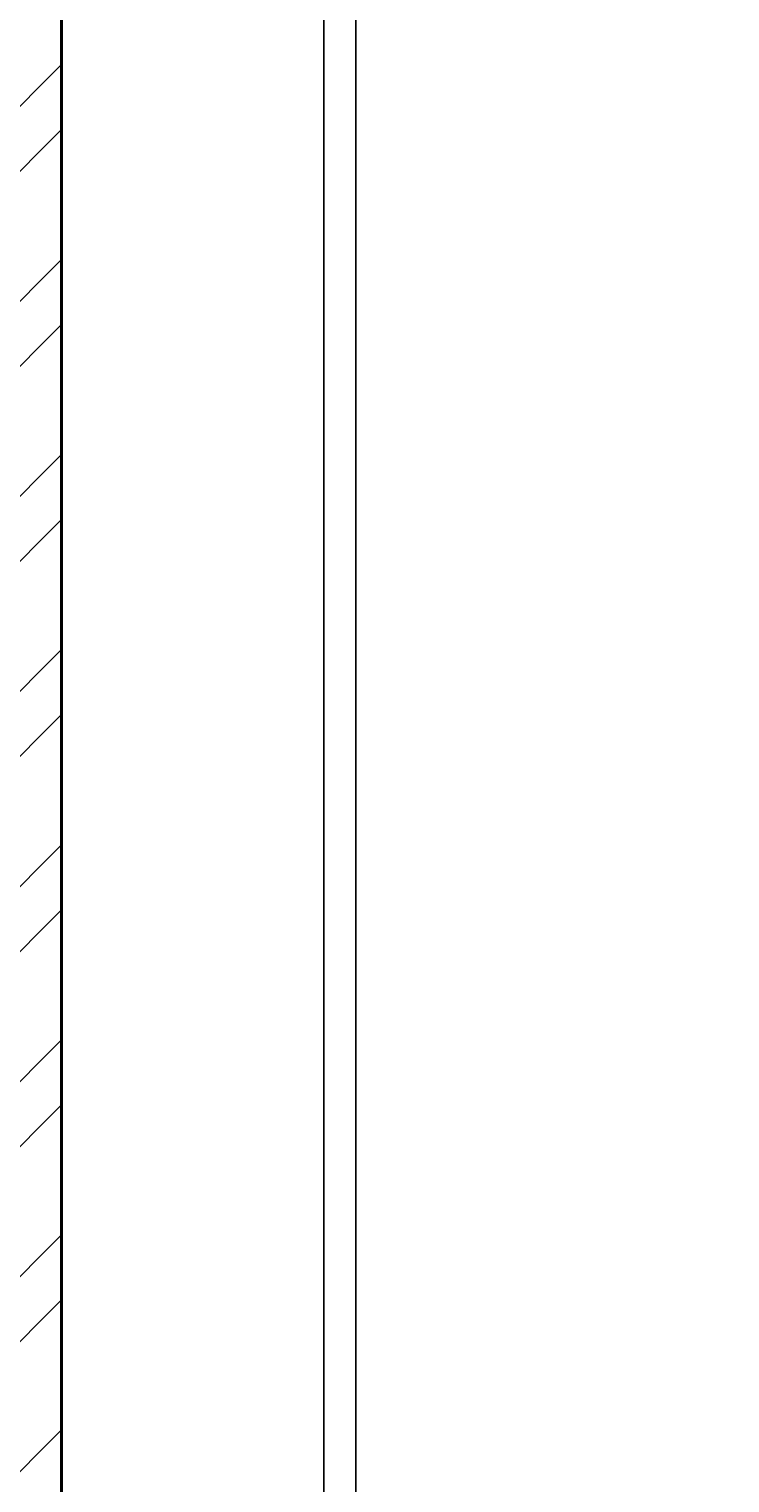
# Model space of a CAD drawing. Units: inches. Extents: x 2063 to 2617, y 1299 to 2210.
# Tile 16 of 22: x 2338 to 2387, y 1839 to 1939. Entities that reach past the tile are written whole.
import ezdxf

# ---------------------------------------------------------------- set-up
doc = ezdxf.new("R2010")
doc.units = ezdxf.units.IN
doc.layers.add('A-ANNO-DIMS', color=2, linetype='Continuous', lineweight=18)
doc.layers.add('A-WALL', color=7, linetype='Continuous', lineweight=40)
doc.layers.add('A-WALL-PATT', color=215, linetype='Continuous', lineweight=13, true_color=0xa953a0)
doc.styles.get("Standard").update_dxf_attribs({"font": 'arial.ttf'})
doc.dimstyles.get("Standard").update_dxf_attribs({"dimtxt": 0.18, "dimasz": 0.18, "dimexe": 0.18, "dimexo": 0.0625, "dimgap": 0.09, "dimtad": 0, "dimtih": 1, "dimtoh": 1, "dimdec": 4, "dimzin": 0, "dimdsep": 46, "dimtxsty": 'Standard', "dimcen": 0.09, "dimadec": 0, "dimazin": 0, "dimtfac": 1, "dimtdec": 4, "dimtofl": 0, "dimtmove": 0, "dimatfit": 3, "dimfxl": 1, "dimtolj": 1, "dimtzin": 0, "dimarcsym": 0})

# ---------------------------------------------------------------- blocks, each defined once
blk = doc.blocks.new('*D51')
at = {"layer": 'A-ANNO-DIMS', "color": 0, "lineweight": -2, "transparency": 16777216}
for p, q in [((2340.64, 2124.25), (2340.64, 1317.7)), ((2358.75, 2124.25), (2358.75, 1317.7)), ((2340.82, 1317.88), (2349.24, 1317.88)), ((2358.57, 1317.88), (2350.15, 1317.88))]:
    blk.add_line(p, q, dxfattribs=at)
at = {"layer": 'A-ANNO-DIMS', "color": 0, "transparency": 16777216}
for points in [[(2340.82, 1317.91), (2340.82, 1317.85), (2340.64, 1317.88)], [(2358.57, 1317.91), (2358.57, 1317.85), (2358.75, 1317.88)]]:
    blk.add_solid(points, dxfattribs=at)
at = {"layer": 'Defpoints', "color": 0, "transparency": 16777216}
for p in [(2340.64, 2124.31), (2358.75, 2124.31), (2358.75, 1317.88)]:
    blk.add_point(p, dxfattribs=at)
at = {"layer": 'A-ANNO-DIMS', "color": 0, "transparency": 16777216, "insert": (2349.7, 1317.88), "char_height": 0.18, "attachment_point": 5}
blk.add_mtext('\\A1;18.106', dxfattribs=at)
blk = doc.blocks.new('*D54')
at = {"layer": 'A-ANNO-DIMS', "color": 0, "lineweight": -2, "transparency": 16777216}
for p, q in [((2340.64, 2124.25), (2340.64, 1317.7)), ((2360.96, 2104.46), (2360.96, 1317.7)), ((2340.82, 1317.88), (2350.34, 1317.88)), ((2360.78, 1317.88), (2351.27, 1317.88))]:
    blk.add_line(p, q, dxfattribs=at)
at = {"layer": 'A-ANNO-DIMS', "color": 0, "transparency": 16777216}
for points in [[(2340.82, 1317.91), (2340.82, 1317.85), (2340.64, 1317.88)], [(2360.78, 1317.91), (2360.78, 1317.85), (2360.96, 1317.88)]]:
    blk.add_solid(points, dxfattribs=at)
at = {"layer": 'Defpoints', "color": 0, "transparency": 16777216}
for p in [(2340.64, 2124.31), (2360.96, 2104.52), (2360.96, 1317.88)]:
    blk.add_point(p, dxfattribs=at)
at = {"layer": 'A-ANNO-DIMS', "color": 0, "transparency": 16777216, "insert": (2350.8, 1317.88), "char_height": 0.18, "attachment_point": 5}
blk.add_mtext('\\A1;20.317', dxfattribs=at)
blk = doc.blocks.new('*D59')
at = {"layer": 'A-ANNO-DIMS', "color": 0, "lineweight": -2, "transparency": 16777216}
for p, q in [((2290.14, 1554.56), (2290.14, 2170.74)), ((2290.32, 2170.56), (2315.07, 2170.56)), ((2340.46, 2170.56), (2315.72, 2170.56)), ((2340.64, 1554.56), (2340.64, 2170.74))]:
    blk.add_line(p, q, dxfattribs=at)
at = {"layer": 'A-ANNO-DIMS', "color": 0, "transparency": 16777216}
for points in [[(2290.32, 2170.59), (2290.32, 2170.53), (2290.14, 2170.56)], [(2340.46, 2170.59), (2340.46, 2170.53), (2340.64, 2170.56)]]:
    blk.add_solid(points, dxfattribs=at)
at = {"layer": 'Defpoints', "color": 0, "transparency": 16777216}
for p in [(2340.64, 2170.56), (2290.14, 1554.5), (2340.64, 1554.5)]:
    blk.add_point(p, dxfattribs=at)
at = {"layer": 'A-ANNO-DIMS', "color": 0, "transparency": 16777216, "insert": (2315.39, 2170.56), "char_height": 0.18, "attachment_point": 5}
blk.add_mtext('\\A1;50.5', dxfattribs=at)

msp = doc.modelspace()

# ---------------------------------------------------------------- hatches: boundary and pattern name
at = {"layer": 'A-WALL-PATT'}
h = msp.add_hatch(dxfattribs=at)
h.set_pattern_fill('ANSI32', color=256)
h.paths.add_polyline_path([(2553.6442, 2128.8122), (2511.1703, 2128.8122), (2511.1703, 2124.3122), (2549.1442, 2124.3122), (2549.1442, 2095.662), (2553.6442, 2095.662)])
h.paths.add_polyline_path([(2553.6442, 2035.662), (2549.1442, 2035.662), (2549.1442, 1980.3122), (2503.7214, 1980.3122), (2503.7214, 1975.8122), (2549.1442, 1975.8122), (2549.1442, 1962.9693), (2553.6442, 1962.9693)])
h.paths.add_polyline_path([(2553.6442, 1938.9693), (2549.1442, 1938.9693), (2549.1442, 1927.8122), (2477.1442, 1927.8122), (2477.1442, 1975.8122), (2481.2918, 1975.8122), (2481.2918, 1980.3122), (2453.2648, 1980.3122), (2453.2648, 1975.8122), (2472.6442, 1975.8122), (2472.6442, 1868.3122), (2400.6442, 1868.3122), (2400.6442, 1861.3782), (2405.1442, 1861.3782), (2405.1442, 1863.8122), (2480.9699, 1863.8122), (2480.9699, 1866.0622), (2480.9699, 1868.3122), (2477.1442, 1868.3122), (2477.1442, 1923.3122), (2549.1442, 1923.3122), (2549.1442, 1908.8504), (2553.6442, 1908.8504)])
h.paths.add_polyline_path([(2553.6442, 1884.8504), (2549.1442, 1884.8504), (2549.1442, 1868.3122), (2501.0636, 1868.3122), (2501.0636, 1863.8122), (2549.1442, 1863.8122), (2549.1442, 1826.0298), (2553.6442, 1826.0298)])
h.paths.add_polyline_path([(2388.1504, 1980.3122), (2340.6442, 1980.3122), (2340.6442, 2124.3122), (2358.7501, 2124.3122), (2358.7501, 2128.8122), (2316.3482, 2128.8122), (2316.3482, 2124.3122), (2336.1442, 2124.3122), (2336.1442, 1980.3122), (2289.1737, 1980.3122), (2289.1737, 1975.8122), (2336.1442, 1975.8122), (2336.1442, 1619.3122), (2333.1433, 1619.3122), (2333.1433, 1614.8122), (2344.1671, 1614.8122), (2344.1671, 1617.0622), (2344.1671, 1619.3122), (2340.6442, 1619.3122), (2340.6442, 1975.8122), (2388.1504, 1975.8122), (2388.1504, 1978.0622)])
h.paths.add_polyline_path([(2290.1442, 1614.8122), (2301.4594, 1614.8122), (2301.4594, 1617.0622), (2301.4594, 1619.3122), (2285.6442, 1619.3122), (2285.6442, 1566.8122), (2280.8619, 1566.8122), (2280.8619, 1564.5622), (2280.8619, 1562.3122), (2285.6442, 1562.3122), (2285.6442, 1442.3122), (2281.7879, 1442.3122), (2281.7879, 1437.8122), (2285.6442, 1437.8122), (2285.6442, 1401.8122), (2290.1442, 1401.8122)])
h.paths.add_polyline_path([(2549.1442, 1731.8122), (2405.1442, 1731.8122), (2405.1442, 1834.4638), (2402.8942, 1834.4638), (2400.6442, 1834.4638), (2400.6442, 1727.3122), (2549.1442, 1727.3122)])
h.paths.add_polyline_path([(2553.6442, 1766.0298), (2551.3942, 1766.0298), (2549.1442, 1766.0298), (2549.1442, 1686.7767), (2553.6442, 1686.7767)])
h.paths.add_polyline_path([(2553.6442, 1638.7767), (2551.3942, 1638.7767), (2549.1442, 1638.7767), (2549.1442, 1619.3122), (2448.6442, 1619.3122), (2448.6442, 1610.5671), (2450.8942, 1610.5671), (2453.1442, 1610.5671), (2453.1442, 1614.8122), (2549.1442, 1614.8122), (2549.1442, 1601.6421), (2553.6442, 1601.6421)])
h.paths.add_polyline_path([(2553.6442, 1577.6421), (2551.3942, 1577.6421), (2549.1442, 1577.6421), (2549.1442, 1566.8122), (2453.1442, 1566.8122), (2453.1442, 1591.5045), (2451.0335, 1591.5045), (2448.6442, 1591.5045), (2448.6442, 1566.8122), (2434.0475, 1566.8122), (2434.0475, 1562.3122), (2549.1442, 1562.3122), (2549.1442, 1533.48), (2553.6442, 1533.48)])
h.paths.add_polyline_path([(2553.6442, 1473.48), (2549.1442, 1473.48), (2549.1442, 1442.3122), (2502.6258, 1442.3122), (2502.6258, 1437.8122), (2549.1442, 1437.8122), (2549.1442, 1401.8122), (2553.6442, 1401.8122)])
h.paths.add_polyline_path([(2395.6442, 1562.3122), (2400.0901, 1562.3122), (2400.0901, 1564.5622), (2400.0901, 1566.8122), (2395.6442, 1566.8122), (2395.6442, 1619.3122), (2379.1127, 1619.3122), (2379.1127, 1614.8122), (2391.1442, 1614.8122), (2391.1442, 1401.8122), (2395.6442, 1401.8122), (2395.6442, 1437.8122), (2399.2425, 1437.8122), (2399.2425, 1440.0622), (2399.2425, 1442.3122), (2395.6442, 1442.3122)])
h.paths.add_polyline_path([(2442.6258, 1442.3122), (2419.6262, 1442.3122), (2419.6262, 1437.8122), (2442.6258, 1437.8122), (2442.6258, 1440.0622)])
h.paths.add_polyline_path([(2127.6442, 1480.2532), (2125.3942, 1480.2532), (2123.1442, 1480.2532), (2123.1442, 1401.8122), (2127.6442, 1401.8122), (2127.6442, 1437.8122), (2145.1538, 1437.8122), (2145.1538, 1440.0622), (2145.1538, 1442.3122), (2127.6442, 1442.3122)])
h.paths.add_polyline_path([(2259.809, 1442.3122), (2205.1538, 1442.3122), (2205.1538, 1437.8122), (2259.809, 1437.8122), (2259.809, 1440.0622)])
h.paths.add_polyline_path([(2127.6442, 1659.7652), (2123.1442, 1659.7652), (2123.1442, 1605.5161), (2125.3942, 1605.5161), (2127.6442, 1605.5161), (2127.6442, 1614.8122), (2223.6442, 1614.8122), (2223.6442, 1611.2723), (2228.1442, 1611.2723), (2228.1442, 1619.3122), (2127.6442, 1619.3122)])
h.paths.add_polyline_path([(2244.8673, 1566.8122), (2228.1442, 1566.8122), (2228.1442, 1590.8122), (2225.8942, 1590.8122), (2223.6442, 1590.8122), (2223.6442, 1566.8122), (2127.6442, 1566.8122), (2127.6442, 1581.5161), (2123.1442, 1581.5161), (2123.1442, 1540.2532), (2127.6442, 1540.2532), (2127.6442, 1562.3122), (2244.8673, 1562.3122), (2244.8673, 1564.5622)])
h.paths.add_polyline_path([(2172.5174, 1868.3122), (2127.6442, 1868.3122), (2127.6442, 1886.5833), (2123.1442, 1886.5833), (2123.1442, 1832.6633), (2127.6442, 1832.6633), (2127.6442, 1863.8122), (2172.5174, 1863.8122), (2172.5174, 1866.0622)])
h.paths.add_polyline_path([(2276.1442, 1868.3122), (2204.1442, 1868.3122), (2204.1442, 1923.3122), (2204.1442, 1975.8122), (2224.8362, 1975.8122), (2224.8362, 1978.1097), (2224.8362, 1980.3122), (2195.0729, 1980.3122), (2195.0729, 1978.0622), (2195.0729, 1975.8122), (2199.6442, 1975.8122), (2199.6442, 1927.8122), (2127.6442, 1927.8122), (2127.6442, 1942.3492), (2123.1442, 1942.3492), (2123.1442, 1910.5833), (2127.6442, 1910.5833), (2127.6442, 1923.3122), (2199.6442, 1923.3122), (2199.6442, 1868.3122), (2194.8228, 1868.3122), (2194.8228, 1864.7337), (2194.8228, 1863.8122), (2271.6442, 1863.8122), (2271.6442, 1860.0507), (2276.1442, 1860.0507)])
h.paths.add_polyline_path([(2276.1442, 1829.994), (2273.8942, 1829.994), (2271.6442, 1829.994), (2271.6442, 1731.8122), (2127.6442, 1731.8122), (2127.6442, 1772.6633), (2123.1442, 1772.6633), (2123.1442, 1707.7652), (2127.6442, 1707.7652), (2127.6442, 1727.3122), (2276.1442, 1727.3122)])
h.paths.add_polyline_path([(2127.6442, 2022.1152), (2123.1442, 2022.1152), (2123.1442, 1966.3492), (2127.6442, 1966.3492), (2127.6442, 1975.8122), (2174.2082, 1975.8122), (2174.2082, 1978.0622), (2174.2082, 1980.3122), (2127.6442, 1980.3122)])
h.paths.add_polyline_path([(2361.9755, 1678.588), (2398.4558, 1678.588), (2398.4558, 1697.2453), (2361.9755, 1697.2453)], flags=9)
h.paths.add_polyline_path([(2351.5397, 1780.4072), (2386.1987, 1780.4072), (2386.1987, 1790.7107), (2351.5397, 1790.7107)], flags=25)
h.paths.add_polyline_path([(2350.6753, 1940.9321), (2387.6024, 1940.9321), (2387.6024, 1959.5894), (2350.6753, 1959.5894)], flags=25)
h.paths.add_polyline_path([(2254.9545, 1684.638), (2295.0943, 1684.638), (2295.0943, 1703.2953), (2254.9545, 1703.2953)], flags=9)
h.paths.add_polyline_path([(2282.4946, 1782.4438), (2317.1535, 1782.4438), (2317.1535, 1792.7474), (2282.4946, 1792.7474)], flags=9)
h.paths.add_polyline_path([(2270.327, 1939.2854), (2307.254, 1939.2854), (2307.254, 1957.9428), (2270.327, 1957.9428)], flags=9)

# ---------------------------------------------------------------- linework, layer by layer
at = {"layer": 'A-WALL'}
msp.add_line((2340.6442, 1975.8122), (2340.6442, 1619.3122), dxfattribs=at)

# ---------------------------------------------------------------- dimensions: what is measured, and where the dimension line sits
at = {"layer": 'A-ANNO-DIMS'}
for base, p1, p2, override, picture, middle in [((2340.6442, 2170.5622), (2290.1442, 1554.4994), (2340.6442, 1554.4994), {"dimdec": 1, "dimlfac": 1, "dimrnd": 0, "dimzin": 0, "dimdsep": 46, "dimlunit": 2}, '*D59', (2315.3942, 2170.5622)), ((2358.7501, 1317.8821), (2340.6442, 2124.3122), (2358.7501, 2124.3122), {"dimdec": 3, "dimlfac": 1, "dimrnd": 0, "dimzin": 0, "dimdsep": 46, "dimlunit": 2}, '*D51', (2349.6972, 1317.8821)), ((2360.9612, 1317.8821), (2340.6442, 2124.3122), (2360.9612, 2104.5201), {"dimdec": 3, "dimlfac": 1, "dimrnd": 0, "dimzin": 0, "dimdsep": 46, "dimlunit": 2}, '*D54', (2350.8027, 1317.8821))]:
    dim = msp.add_linear_dim(base=base, p1=p1, p2=p2, dimstyle='Standard', override=override, dxfattribs=at)
    dim.commit()
    dim.dimension.update_dxf_attribs({"geometry": picture, "text_midpoint": middle})

doc.saveas('drawing.dxf')
